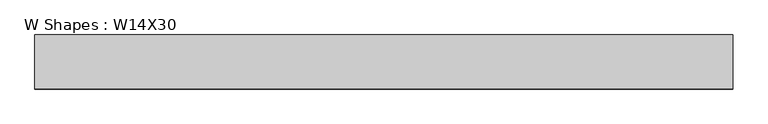
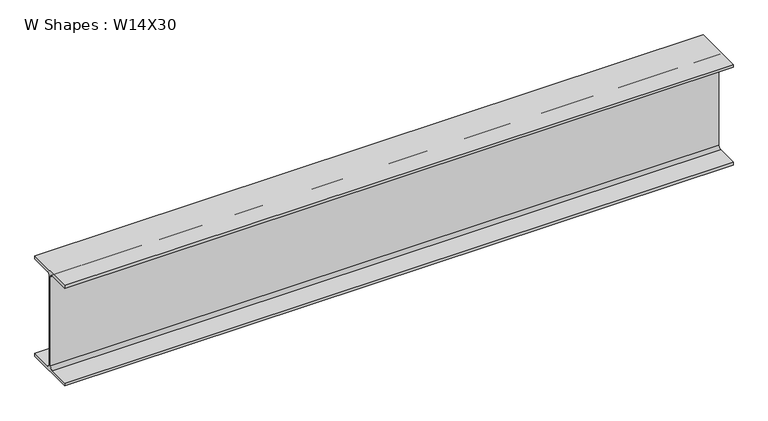
"""IFC4 building model written with IfcOpenShell, lengths in millimetres: beam geometry, W Shapes : W14X30."""

from ifc_helpers import new_model, si_unit, point, frame, frame_2d, origin, place, context, project, spatial, polyline, circle_curve, trimmed, segment, composite_curve, outline, extrude, source, transform, mapped, element, save


def w_shapes_w14x30_333ad3b1(model_context):
    return source(origin(), model_context, "Body", "SweptSolid", [
        extrude(outline(composite_curve([segment(polyline([(85.471, -165.481), (85.471, -175.26), (-85.471, -175.26), (-85.471, -165.481), (-13.589, -165.481)]), True, "CONTINUOUS"), segment(trimmed(circle_curve(frame_2d((-13.589, -155.321)), 10.16), [point((-13.589, -165.481))], [point((-3.429, -155.321))], True, "CARTESIAN"), True, "CONTINUOUS"), segment(polyline([(-3.429, -155.321), (-3.429, 155.321)]), True, "CONTINUOUS"), segment(trimmed(circle_curve(frame_2d((-13.589, 155.321)), 10.16), [point((-3.429, 155.321))], [point((-13.589, 165.481))], True, "CARTESIAN"), True, "CONTINUOUS"), segment(polyline([(-13.589, 165.481), (-85.471, 165.481), (-85.471, 175.26), (85.471, 175.26), (85.471, 165.481), (13.589, 165.481)]), True, "CONTINUOUS"), segment(trimmed(circle_curve(frame_2d((13.589, 155.321)), 10.16), [point((13.589, 165.481))], [point((3.429, 155.321))], True, "CARTESIAN"), True, "CONTINUOUS"), segment(polyline([(3.429, 155.321), (3.429, -155.321)]), True, "CONTINUOUS"), segment(trimmed(circle_curve(frame_2d((13.589, -155.321)), 10.16), [point((3.429, -155.321))], [point((13.589, -165.481))], True, "CARTESIAN"), True, "CONTINUOUS"), segment(polyline([(13.589, -165.481), (85.471, -165.481)]), True, "CONTINUOUS")], self_intersect=False)), frame((-1240.2460849, 0.0, 0.0), z_axis=(1.0, 0.0, 0.0), x_axis=(0.0, 1.0, 0.0)), (0.0, 0.0, 1.0), 2206.7425597),
    ])


if __name__ == "__main__":
    model = new_model("IFC4")
    model_context = context("Model", 3, world=origin())
    ifc_project = project(units=[si_unit("LENGTHUNIT", "METRE", prefix="MILLI")], contexts=[model_context])
    site = spatial("IfcSite", under=ifc_project)
    building = spatial("IfcBuilding", under=site)
    placement = place(None, origin())
    w_shapes_w14x30_shape = w_shapes_w14x30_333ad3b1(model_context)
    element("IfcBeam", 1, ObjectType="W Shapes : W14X30", at=placement, inside=building, context=model_context, shape_type="MappedRepresentation", body=[
        mapped(w_shapes_w14x30_shape, transform((0.0, 0.0, 0.0), x_axis=(1.0, 0.0, 0.0), y_axis=(0.0, 1.0, 0.0), z_axis=(0.0, 0.0, 1.0))),
    ])
    save(model, "model.ifc")

# Revit data of these elements
# Type "W Shapes : W14X30"
#   Section Name Key = "W14X30"
#   Width = 6.730"
#   Web Thickness = 0.270"
#   Web Fillet = 0.400"
#   Warping Constant = 887.00 in⁶
#   Torsional Moment of Inertia = 0.38 in⁴
#   Section Area = 8.85 in²
#   Plastic Modulus weak axis = 8.99 in³
#   Plastic Modulus strong axis = 47.30 in³
#   Perimeter = 4.441 ft²/ft
#   Nominal Weight = 30.00 lbf/ft
#   Moment of Inertia weak axis = 19.60 in⁴
#   Moment of Inertia strong axis = 291.00 in⁴
#   Height = 13.800"
#   Flange Thickness = 0.385"
#   Elastic Modulus weak axis = 5.82 in³
#   Elastic Modulus strong axis = 42.00 in³
#   Clear Web Height = 0' - 11 5/8"
#   Centroid Vertical = 6.900"
#   Centroid Horizontal = 3.365"
#   Bolt Spacing = 0' - 3 1/2"
#   Length [instance default] = 1524 mm
#   Structural Material [instance default] = Steel ASTM A992
#   Principal Axes Angle = 0
# Element 1 (IfcBeam, "W Shapes : W14X30")
#   Length = 3476.809 mm
#   Materials on its faces: "Steel ASTM A992"
# Materials
#   "Steel ASTM A992": class "Metal", colour RGB 199 199 199, transparency 0, Description = "Structural steel 50ksi", Cost = 0
